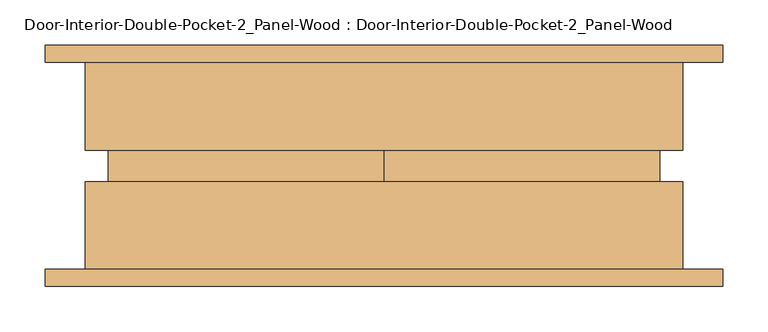
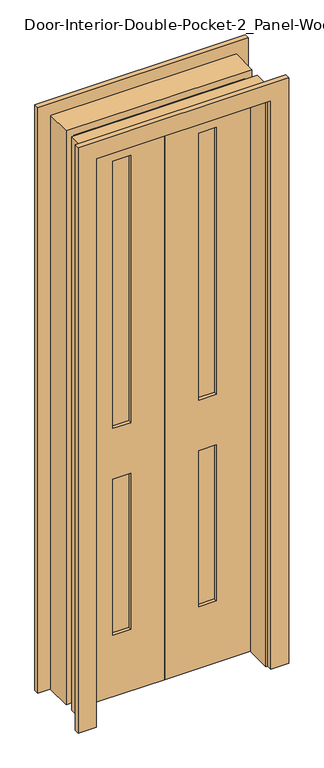
"""IFC4 building model written with IfcOpenShell, lengths in millimetres: door geometry, Door-Interior-Double-Pocket-2_Panel-Wood : Door-Interior-Double-Pocket-2_Panel-Wood."""

from ifc_helpers import new_model, si_unit, frame, origin, place, context, project, spatial, polyline, outline, extrude, source, transform, mapped, element, save


def door_interior_double_pocket_2_panel_wood_door_interior_52fbc1e8(model_context):
    return source(origin(), model_context, "Body", "SweptSolid", [
        extrude(outline(polyline([(0.0, 311.15), (0.0, 374.65), (2203.45, 374.65), (2203.45, -374.65), (0.0, -374.65), (0.0, -311.15), (2139.95, -311.15), (2139.95, 311.15), (0.0, 311.15)])), frame((0.0, 114.3, 0.0), z_axis=(0.0, 1.0, 0.0), x_axis=(0.0, 0.0, 1.0)), (0.0, 0.0, 1.0), 19.05),
        extrude(outline(polyline([(0.0, 311.15), (0.0, 374.65), (2203.45, 374.65), (2203.45, -374.65), (0.0, -374.65), (0.0, -311.15), (2139.95, -311.15), (2139.95, 311.15), (0.0, 311.15)])), frame((0.0, -133.35, 0.0), z_axis=(0.0, 1.0, 0.0), x_axis=(0.0, 0.0, 1.0)), (0.0, 0.0, 1.0), 19.05),
        extrude(outline(polyline([(2133.6, 0.0), (0.0, 0.0), (0.0, 304.8), (2133.6, 304.8), (2133.6, 0.0)]), holes=[polyline([(2014.5375, 120.65), (2014.5375, 184.15), (1009.65, 184.15), (1009.65, 120.65), (2014.5375, 120.65)]), polyline([(819.15, 120.65), (819.15, 184.15), (231.775, 184.15), (231.775, 120.65), (819.15, 120.65)])]), frame((0.0, -17.4625, 0.0), z_axis=(0.0, 1.0, 0.0), x_axis=(0.0, 0.0, 1.0)), (0.0, 0.0, 1.0), 34.925),
        extrude(outline(polyline([(184.15, -5.8208333), (120.65, -5.8208333), (120.65, 5.8208333), (184.15, 5.8208333), (184.15, -5.8208333)])), frame((0.0, 0.0, 1009.65), z_axis=(0.0, 0.0, 1.0), x_axis=(1.0, 0.0, 0.0)), (0.0, 0.0, 1.0), 1004.8875),
        extrude(outline(polyline([(184.15, -5.8208333), (120.65, -5.8208333), (120.65, 5.8208333), (184.15, 5.8208333), (184.15, -5.8208333)])), frame((0.0, 0.0, 231.775), z_axis=(0.0, 0.0, 1.0), x_axis=(1.0, 0.0, 0.0)), (0.0, 0.0, 1.0), 587.375),
        extrude(outline(polyline([(0.0, 330.2), (2159.0, 330.2), (2159.0, -330.2), (0.0, -330.2), (0.0, -304.8), (2133.6, -304.8), (2133.6, 304.8), (0.0, 304.8), (0.0, 330.2)])), frame((0.0, 17.4625, 0.0), z_axis=(0.0, 1.0, 0.0), x_axis=(0.0, 0.0, 1.0)), (0.0, 0.0, 1.0), 96.8375),
        extrude(outline(polyline([(0.0, 330.2), (2159.0, 330.2), (2159.0, -330.2), (0.0, -330.2), (0.0, -304.8), (2133.6, -304.8), (2133.6, 304.8), (0.0, 304.8), (0.0, 330.2)])), frame((0.0, -114.3, 0.0), z_axis=(0.0, 1.0, 0.0), x_axis=(0.0, 0.0, 1.0)), (0.0, 0.0, 1.0), 96.8375),
        extrude(outline(polyline([(2133.6, -304.8), (0.0, -304.8), (0.0, 0.0), (2133.6, 0.0), (2133.6, -304.8)]), holes=[polyline([(2014.5375, -184.15), (2014.5375, -120.65), (1009.65, -120.65), (1009.65, -184.15), (2014.5375, -184.15)]), polyline([(819.15, -184.15), (819.15, -120.65), (231.775, -120.65), (231.775, -184.15), (819.15, -184.15)])]), frame((0.0, -17.4625, 0.0), z_axis=(0.0, 1.0, 0.0), x_axis=(0.0, 0.0, 1.0)), (0.0, 0.0, 1.0), 34.925),
        extrude(outline(polyline([(-120.65, -5.8208333), (-184.15, -5.8208333), (-184.15, 5.8208333), (-120.65, 5.8208333), (-120.65, -5.8208333)])), frame((0.0, 0.0, 1009.65), z_axis=(0.0, 0.0, 1.0), x_axis=(1.0, 0.0, 0.0)), (0.0, 0.0, 1.0), 1004.8875),
        extrude(outline(polyline([(-120.65, -5.8208333), (-184.15, -5.8208333), (-184.15, 5.8208333), (-120.65, 5.8208333), (-120.65, -5.8208333)])), frame((0.0, 0.0, 231.775), z_axis=(0.0, 0.0, 1.0), x_axis=(1.0, 0.0, 0.0)), (0.0, 0.0, 1.0), 587.375),
    ])


if __name__ == "__main__":
    model = new_model("IFC4")
    model_context = context("Model", 3, world=origin())
    ifc_project = project(units=[si_unit("LENGTHUNIT", "METRE", prefix="MILLI")], contexts=[model_context])
    site = spatial("IfcSite", under=ifc_project)
    building = spatial("IfcBuilding", under=site)
    placement = place(None, origin())
    door_interior_double_pocket_2_panel_wood_door_interior_shape = door_interior_double_pocket_2_panel_wood_door_interior_52fbc1e8(model_context)
    element("IfcDoor", 1, ObjectType="Door-Interior-Double-Pocket-2_Panel-Wood : Door-Interior-Double-Pocket-2_Panel-Wood", at=placement, inside=building, context=model_context, shape_type="MappedRepresentation", body=[
        mapped(door_interior_double_pocket_2_panel_wood_door_interior_shape, transform((0.0, 0.0, 0.0), x_axis=(1.0, 0.0, 0.0), y_axis=(0.0, 1.0, 0.0), z_axis=(0.0, 0.0, 1.0))),
    ])
    save(model, "model.ifc")

# Revit data of these elements
# Type "Door-Interior-Double-Pocket-2_Panel-Wood : Door-Interior-Double-Pocket-2_Panel-Wood"
#   Type Mark = "14"
#   Assembly Code = "C1020300"
#   Analytic Construction = "Wooden"
#   Top Rail = 0' - 4 11/16"
#   Thickness = 0' - 1 3/8"
#   Thermal Resistance (R) = 2.5876 (h·ft²·°F)/BTU
#   Stiles = 0' - 4 3/4"
#   Rough Width = 4' - 2"
#   Rough Height = 7' - 4 1/2"
#   Panel Width = 1' - 0"
#   Lock Rail = 0' - 7 1/2"
#   Location [instance default] = 1' - 1"
#   Height = 7' - 0"
#   Width = 2' - 0"
#   Heat Transfer Coefficient (U) = 0.3865 BTU/(h·ft²·°F)
#   Bottom Rail = 0' - 9 1/8"
#   Panel Open [instance default] = no
#   Trim Material = Cherry
#   Panel Material = Cherry
#   Frame Material = Cherry
#   Visual Light Transmittance = 0
#   Solar Heat Gain Coefficient = 0
#   Wall Closure = (empty or 0)
#   Function = (empty or 0)
# Element 1 (IfcDoor, "Door-Interior-Double-Pocket-2_Panel-Wood : Door-Interior-Double-Pocket-2_Panel-Wood")
#   Materials on its faces: "Cherry"
# Materials
#   "Cherry": class "Wood", colour RGB 226 177 128, transparency 0, Description = "Prunus Serotina", Cost = 0
